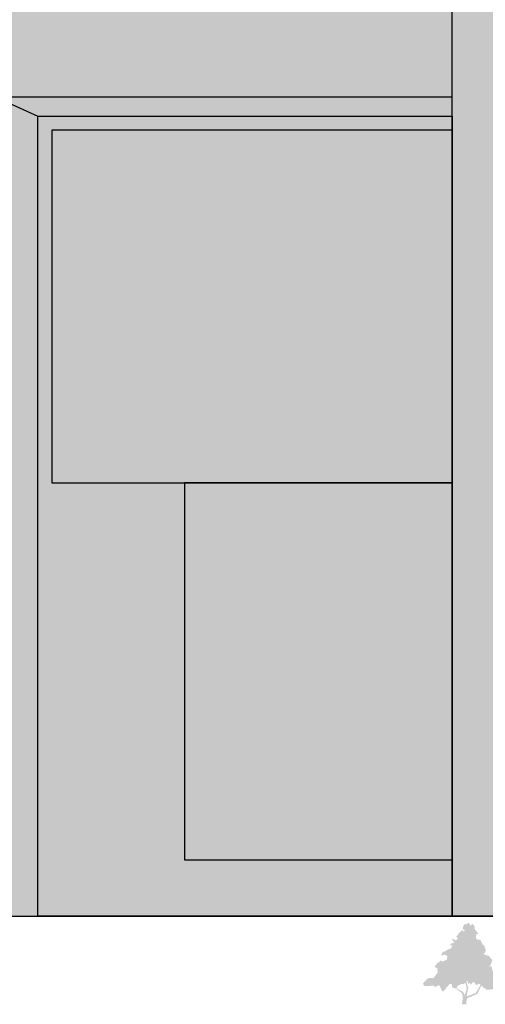
# Model space of a CAD drawing. Units: feet. Extents: x 2368 to 3224, y 836 to 1229.
# Tile 5 of 9: x 2447 to 2515, y 841 to 985. Entities that reach past the tile are written whole.
import ezdxf

# ---------------------------------------------------------------- set-up
doc = ezdxf.new("R2010")
doc.units = ezdxf.units.FT
for name, color, linetype, lineweight in [('A-ELEV', 7, 'Continuous', 25), ('A-ELEV-PATT', 8, 'Continuous', 13), ('L-PLNT', 3, 'Continuous', 13)]:
    doc.layers.add(name, color=color, linetype=linetype, lineweight=lineweight)

msp = doc.modelspace()

# ---------------------------------------------------------------- hatches: boundary and pattern name
at = {"layer": 'A-ELEV-PATT'}
h = msp.add_hatch(color=256, dxfattribs=at)
h.dxf.hatch_style = 1
h.paths.add_polyline_path([(2582.11, 1191.22), (2544.98, 1191.22), (2544.98, 1108.75), (2582.11, 1108.75)])
h.paths.add_polyline_path([(2653.72, 1191.22), (2584.6, 1191.22), (2584.6, 1108.75), (2653.72, 1108.75)])
h.paths.add_polyline_path([(2693.73, 1191.22), (2656.21, 1191.22), (2656.21, 1108.75), (2693.73, 1108.75)])
h.paths.add_polyline_path([(2653.72, 1099.51), (2584.6, 1099.51), (2584.6, 1040.78), (2653.72, 1040.78)])
h.paths.add_polyline_path([(2693.73, 1099.51), (2656.21, 1099.51), (2656.21, 1040.78), (2693.73, 1040.78)])
h.paths.add_polyline_path([(2582.11, 1099.51), (2544.98, 1099.51), (2544.98, 1040.78), (2582.11, 1040.78)])
h.paths.add_polyline_path([(2582.11, 1036.77), (2544.98, 1036.77), (2544.98, 1033.48), (2582.11, 1033.48)])
h.paths.add_polyline_path([(2582.11, 1033.11), (2544.98, 1033.11), (2544.98, 1029.83), (2582.11, 1029.83)])
h.paths.add_polyline_path([(2582.11, 1029.46), (2544.98, 1029.46), (2544.98, 1026.18), (2582.11, 1026.18)])
h.paths.add_polyline_path([(2582.11, 1025.81), (2544.98, 1025.81), (2544.98, 1022.52), (2582.11, 1022.52)])
h.paths.add_polyline_path([(2582.11, 1022.15), (2544.98, 1022.15), (2544.98, 1018.87), (2582.11, 1018.87)])
h.paths.add_polyline_path([(2582.11, 1018.5), (2544.98, 1018.5), (2544.98, 1015.21), (2582.11, 1015.21)])
h.paths.add_polyline_path([(2582.11, 1007.53), (2544.98, 1007.53), (2544.98, 1006.11), (2582.11, 1006.11)])
h.paths.add_polyline_path([(2582.11, 1011.19), (2544.98, 1011.19), (2544.98, 1007.9), (2582.11, 1007.9)])
h.paths.add_polyline_path([(2582.11, 1014.84), (2544.98, 1014.84), (2544.98, 1011.56), (2582.11, 1011.56)])
h.paths.add_polyline_path([(2619.49, 1007.53), (2584.6, 1007.53), (2584.6, 1006.11), (2619.49, 1006.11)])
h.paths.add_polyline_path([(2619.49, 1011.19), (2584.6, 1011.19), (2584.6, 1007.9), (2619.49, 1007.9)])
h.paths.add_polyline_path([(2619.49, 1014.84), (2584.6, 1014.84), (2584.6, 1011.56), (2619.49, 1011.56)])
h.paths.add_polyline_path([(2619.49, 1018.5), (2584.6, 1018.5), (2584.6, 1015.21), (2619.49, 1015.21)])
h.paths.add_polyline_path([(2619.49, 1022.15), (2584.6, 1022.15), (2584.6, 1018.87), (2619.49, 1018.87)])
h.paths.add_polyline_path([(2619.49, 1025.81), (2584.6, 1025.81), (2584.6, 1022.52), (2619.49, 1022.52)])
h.paths.add_polyline_path([(2619.49, 1029.46), (2584.6, 1029.46), (2584.6, 1026.18), (2619.49, 1026.18)])
h.paths.add_polyline_path([(2619.49, 1033.11), (2584.6, 1033.11), (2584.6, 1029.83), (2619.49, 1029.83)])
h.paths.add_polyline_path([(2619.49, 1036.77), (2584.6, 1036.77), (2584.6, 1033.48), (2619.49, 1033.48)])
h.paths.add_polyline_path([(2582.11, 1040.06), (2544.98, 1040.06), (2544.98, 1037.14), (2582.11, 1037.14)])
h.paths.add_polyline_path([(2619.49, 1040.06), (2584.6, 1040.06), (2584.6, 1037.14), (2619.49, 1037.14)])
h.paths.add_polyline_path([(2653.72, 1040.06), (2620.43, 1040.06), (2620.43, 1037.14), (2653.72, 1037.14)])
h.paths.add_polyline_path([(2653.72, 1036.77), (2620.43, 1036.77), (2620.43, 1033.48), (2653.72, 1033.48)])
h.paths.add_polyline_path([(2653.72, 1033.11), (2620.43, 1033.11), (2620.43, 1029.83), (2653.72, 1029.83)])
h.paths.add_polyline_path([(2653.72, 1029.46), (2620.43, 1029.46), (2620.43, 1026.18), (2653.72, 1026.18)])
h.paths.add_polyline_path([(2653.72, 1025.81), (2620.43, 1025.81), (2620.43, 1022.52), (2653.72, 1022.52)])
h.paths.add_polyline_path([(2653.72, 1022.15), (2620.43, 1022.15), (2620.43, 1018.87), (2653.72, 1018.87)])
h.paths.add_polyline_path([(2653.72, 1018.5), (2620.43, 1018.5), (2620.43, 1015.21), (2653.72, 1015.21)])
h.paths.add_polyline_path([(2653.72, 1011.19), (2620.43, 1011.19), (2620.43, 1007.9), (2653.72, 1007.9)])
h.paths.add_polyline_path([(2653.72, 1014.84), (2620.43, 1014.84), (2620.43, 1011.56), (2653.72, 1011.56)])
h.paths.add_polyline_path([(2653.72, 1007.53), (2620.43, 1007.53), (2620.43, 1006.11), (2653.72, 1006.11)])
h.paths.add_polyline_path([(2693.73, 1007.53), (2656.21, 1007.53), (2656.21, 1006.11), (2693.73, 1006.11)])
h.paths.add_polyline_path([(2693.73, 1011.19), (2656.21, 1011.19), (2656.21, 1007.9), (2693.73, 1007.9)])
h.paths.add_polyline_path([(2693.73, 1014.84), (2656.21, 1014.84), (2656.21, 1011.56), (2693.73, 1011.56)])
h.paths.add_polyline_path([(2693.73, 1018.5), (2656.21, 1018.5), (2656.21, 1015.21), (2693.73, 1015.21)])
h.paths.add_polyline_path([(2693.73, 1022.15), (2656.21, 1022.15), (2656.21, 1018.87), (2693.73, 1018.87)])
h.paths.add_polyline_path([(2693.73, 1025.81), (2656.21, 1025.81), (2656.21, 1022.52), (2693.73, 1022.52)])
h.paths.add_polyline_path([(2693.73, 1029.46), (2656.21, 1029.46), (2656.21, 1026.18), (2693.73, 1026.18)])
h.paths.add_polyline_path([(2693.73, 1033.11), (2656.21, 1033.11), (2656.21, 1029.83), (2693.73, 1029.83)])
h.paths.add_polyline_path([(2693.73, 1040.06), (2656.21, 1040.06), (2656.21, 1037.14), (2693.73, 1037.14)])
h.paths.add_polyline_path([(2693.73, 1036.77), (2656.21, 1036.77), (2656.21, 1033.48), (2693.73, 1033.48)])
h.paths.add_polyline_path([(2510.02, 968.65), (2451.35, 968.65), (2451.35, 916.99), (2510.02, 916.99)])
h.paths.add_polyline_path([(2510.02, 916.99), (2470.8, 916.99), (2470.8, 861.76), (2510.02, 861.76)])
h.paths.add_polyline_path([(2650.82, 971.36, 0.250141), (2603.19, 971.36), (2603.19, 926.73), (2650.82, 926.73)])
h.paths.add_polyline_path([(2651.5, 971), (2651.5, 926.73), (2677.6, 926.73, 0.272847)])
h.paths.add_polyline_path([(2677.6, 926.06), (2651.5, 926.06), (2651.5, 854.24), (2677.6, 854.24)])
h.paths.add_polyline_path([(2650.82, 926.06), (2603.19, 926.06), (2603.19, 854.24), (2650.82, 854.24)])
h.paths.add_polyline_path([(2602.51, 971, 0.272847), (2576.42, 926.73), (2602.51, 926.73)])
h.paths.add_polyline_path([(2602.51, 926.06), (2576.42, 926.06), (2576.42, 854.24), (2602.51, 854.24)])
h = msp.add_hatch(color=256, dxfattribs=at)
h.dxf.hatch_style = 1
h.paths.add_polyline_path([(2443.04, 973.51), (2394.91, 973.51), (2394.91, 853.51), (2443.04, 853.51)])
h.paths.add_polyline_path([(2422.21, 920.11), (2422.21, 905.78), (2416.4, 905.78), (2416.4, 920.11)], flags=16)
h.paths.add_polyline_path([(2449.3, 970.69), (2443.04, 973.51), (2443.04, 853.51), (2449.3, 853.51)])
h.paths.add_polyline_path([(2510.02, 987.86), (2368.3, 987.86), (2394.91, 973.51), (2443.04, 973.51), (2510.02, 973.51)])
h.paths.add_polyline_path([(2510.02, 973.51), (2443.04, 973.51), (2449.3, 970.69), (2510.02, 970.69)])
h = msp.add_hatch(color=256, dxfattribs=at)
h.dxf.hatch_style = 1
h.paths.add_polyline_path([(2624.92, 981.22), (2624.92, 981.73, -0.018787), (2629.09, 981.73), (2629.09, 981.22, -0.403049), (2681.53, 926.73), (2681.53, 853.51), (2701.14, 853.51), (2719.16, 853.51), (2719.16, 987.86), (2694.93, 987.86), (2544.98, 987.86), (2510.02, 987.86), (2510.02, 853.51), (2520.58, 853.51), (2520.05, 853.96), (2521, 855.17), (2521.51, 855.27), (2521.73, 855.83), (2522.31, 855.46), (2523.63, 855.92), (2523.84, 857.04), (2523.12, 857.51), (2521.95, 857.23), (2522.6, 858.63), (2522.68, 858.26), (2523.55, 858.73), (2524.28, 859.19), (2524.94, 859.29), (2525.23, 860.22), (2524.5, 860.32), (2525.17, 860.97), (2525.74, 860.88), (2525.67, 861.62), (2525.16, 861.72), (2525.3, 862.09), (2525.67, 862.19), (2526.32, 861.72), (2526.98, 862.19), (2526.47, 863.03), (2526.98, 863.31), (2526.98, 863.59), (2528.51, 865.09), (2528.51, 865.74), (2528.95, 866.58), (2529.53, 866.48), (2530.04, 866.95), (2530.41, 866.77), (2530.48, 866.3), (2530.77, 866.11), (2531.28, 866.67), (2531.86, 866.03), (2532.01, 864.99), (2533.1, 863.68), (2532.52, 863.68), (2532.3, 862.65), (2532.67, 861.9), (2533.18, 861.9), (2533.61, 862), (2534.34, 860.41), (2534.71, 860.41), (2535.29, 858.63), (2534.63, 857.61), (2536.09, 857.14), (2537.26, 855.92), (2536.52, 854.02), (2536.97, 853.96), (2537.09, 853.51), (2572.48, 853.51), (2572.48, 926.73, -0.403049)])
h.paths.add_polyline_path([(2536.7, 926.19), (2536.7, 904.71), (2529.87, 904.71), (2529.87, 926.19)], flags=16)
h = msp.add_hatch(color=256, dxfattribs=at)
h.dxf.hatch_style = 1
h.paths.add_polyline_path([(2470.8, 916.99), (2451.35, 916.99), (2451.35, 968.65), (2510.02, 968.65), (2510.02, 970.69), (2449.3, 970.69), (2449.3, 853.51), (2510.02, 853.51), (2510.02, 861.76), (2470.8, 861.76)])
at = {"layer": 'L-PLNT'}
h = msp.add_hatch(color=256, dxfattribs=at)
h.dxf.hatch_style = 1
h.paths.add_polyline_path([(2515.94, 847.08), (2515.36, 847.68), (2514.64, 847.91), (2514.97, 848.41), (2514.68, 849.29), (2514.5, 849.29), (2514.14, 850.07), (2513.93, 850.03), (2513.67, 850.03), (2513.49, 850.4), (2513.6, 850.9), (2513.89, 850.9), (2513.35, 851.55), (2513.28, 852.06), (2512.99, 852.38), (2512.74, 852.1), (2512.6, 852.19), (2512.56, 852.42), (2512.38, 852.52), (2512.13, 852.29), (2511.84, 852.33), (2511.62, 851.92), (2511.62, 851.55), (2511.91, 851.41), (2511.7, 851.27), (2511.48, 851.46), (2510.87, 850.86), (2510.87, 850.72), (2510.62, 850.58), (2510.69, 850.44), (2510.87, 850.17), (2510.55, 849.94), (2510.22, 850.17), (2510.04, 850.12), (2509.97, 849.94), (2510.22, 849.89), (2510.26, 849.52), (2509.98, 849.57), (2509.65, 849.24), (2510.01, 849.2), (2509.86, 848.74), (2509.54, 848.69), (2509.18, 848.46), (2508.75, 848.23), (2508.71, 848.41), (2508.39, 847.72), (2508.96, 847.86), (2509.32, 847.63), (2509.22, 847.08), (2508.57, 846.85), (2508.28, 847.03), (2508.17, 846.76), (2507.92, 846.71), (2507.71, 846.43), (2507.46, 846.11), (2507.78, 845.83), (2507.99, 845.97), (2507.75, 845.57), (2507.93, 845.59), (2507.9, 845.23), (2507.31, 844.45), (2506.59, 844.41), (2506.27, 844.22), (2505.73, 843.62), (2505.95, 843.25), (2507.28, 843.3), (2507.53, 843.12), (2508.14, 843.39), (2508.57, 842.47), (2508.75, 842.47), (2509.58, 843.48), (2509.83, 843.62), (2510.01, 843.39), (2510.01, 843.07), (2510.29, 842.98), (2510.69, 842.98), (2510.83, 843.3), (2511.3, 843.53), (2511.77, 843.58), (2511.98, 843.76), (2512.02, 843.81), (2512.13, 844.04), (2512.27, 843.94), (2512.38, 843.58), (2512.63, 843.71), (2512.7, 843.62), (2512.78, 843.39), (2513.03, 843.81), (2513.28, 843.81), (2513.39, 843.62), (2513.28, 843.44), (2513.57, 843.53), (2513.67, 843.39), (2513.93, 843.58), (2514.18, 843.48), (2514.68, 842.98), (2514.9, 842.88), (2515.08, 842.7), (2516.59, 842.84), (2516.87, 842.56), (2517.09, 842.65), (2516.51, 843.39), (2516.48, 843.67), (2516.66, 843.94), (2516.33, 844.82), (2516.15, 844.82), (2515.79, 846.11), (2515.43, 846.16), (2515.65, 846.34)])
h = msp.add_hatch(color=256, dxfattribs=at)
h.dxf.hatch_style = 1
h.paths.add_polyline_path([(2512.2, 841.46), (2513.71, 842.1), (2514.32, 843.34), (2514.19, 843.47), (2514.18, 843.44), (2513.49, 842.24), (2512.13, 841.73), (2512.38, 842.88), (2512.13, 843.94), (2512.11, 844.01), (2512.02, 843.81), (2511.98, 843.76), (2511.96, 843.74), (2511.98, 843.71), (2512.16, 842.84), (2511.84, 841.87), (2511.73, 842.24), (2511.45, 842.52), (2510.62, 842.93), (2510.55, 842.98), (2510.37, 842.98), (2511.23, 842.42), (2511.52, 842.06), (2511.59, 841.55), (2511.45, 840.58), (2512.13, 840.58), (2512.09, 840.9)])

# ---------------------------------------------------------------- linework, layer by layer
at = {"layer": 'A-ELEV'}
for p, q in [((2394.91, 973.51), (2510.02, 973.51)), ((2394.91, 973.51), (2510.02, 973.51)), ((2443.04, 973.51), (2449.3, 970.69)), ((2443.04, 973.51), (2449.3, 970.69)), ((2394.91, 853.51), (2521.04, 853.51)), ((2394.91, 853.51), (2521.04, 853.51))]:
    msp.add_line(p, q, dxfattribs=at)
for points in [[(2521.04, 853.51), (2510.02, 853.51), (2510.02, 987.86), (2719.16, 987.86), (2719.16, 853.51), (2537.09, 853.51)], [(2521.04, 853.51), (2510.02, 853.51), (2510.02, 987.86), (2719.16, 987.86), (2719.16, 853.51), (2537.09, 853.51)], [(2510.02, 968.65), (2451.35, 968.65), (2451.35, 916.99)], [(2510.02, 968.65), (2451.35, 968.65), (2451.35, 916.99)], [(2451.35, 916.99), (2510.02, 916.99), (2510.02, 853.51), (2449.3, 853.51), (2449.3, 916.99)], [(2451.35, 916.99), (2510.02, 916.99), (2510.02, 853.51), (2449.3, 853.51), (2449.3, 916.99)], [(2451.35, 916.99), (2482.13, 916.99)], [(2451.35, 916.99), (2482.13, 916.99)]]:
    msp.add_lwpolyline(points, dxfattribs=at)
for points in [[(2449.3, 970.69), (2510.02, 970.69), (2510.02, 853.51), (2449.3, 853.51)], [(2449.3, 970.69), (2510.02, 970.69), (2510.02, 853.51), (2449.3, 853.51)], [(2510.02, 916.99), (2470.8, 916.99), (2470.8, 861.76), (2510.02, 861.76)], [(2510.02, 916.99), (2470.8, 916.99), (2470.8, 861.76), (2510.02, 861.76)]]:
    msp.add_lwpolyline(points, close=True, dxfattribs=at)

doc.saveas('drawing.dxf')
